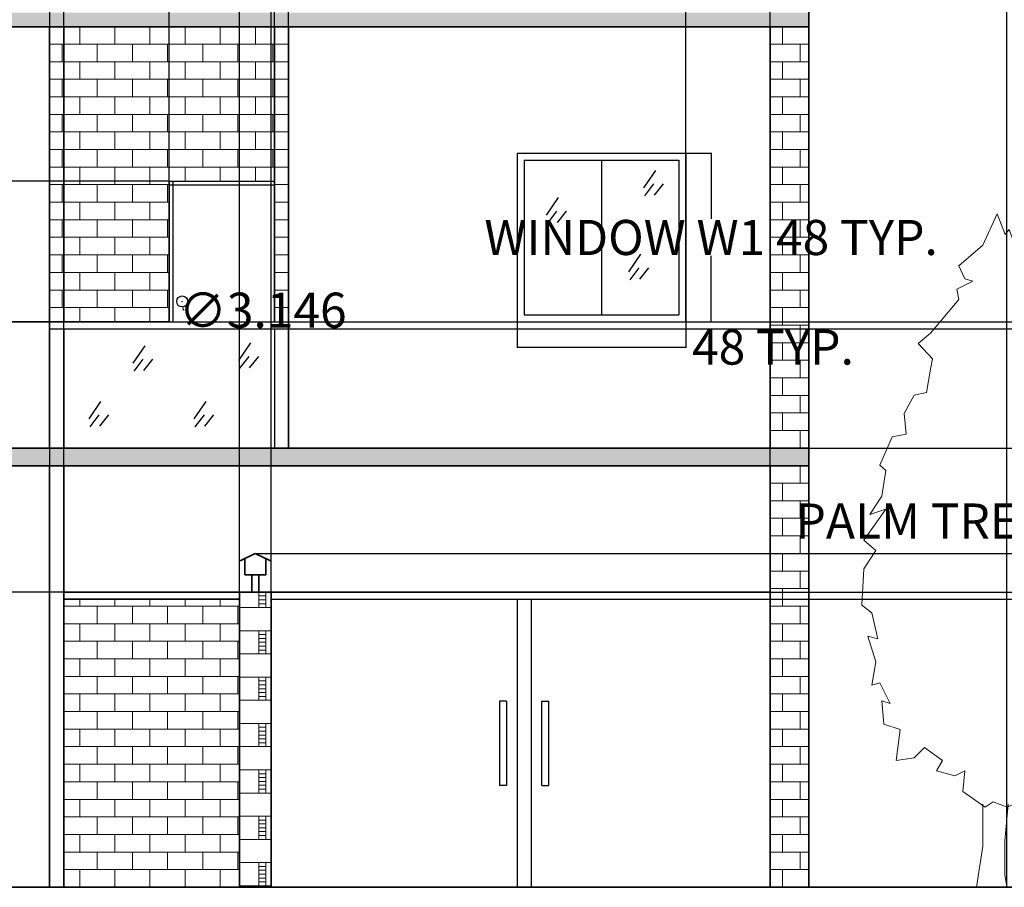
# Model space of a CAD drawing. Units: inches. Extents: x 403 to 1256, y 451 to 842.
# Tile 2 of 4: x 818 to 1098, y 455 to 702. Entities that reach past the tile are written whole.
import ezdxf

# ---------------------------------------------------------------- set-up
doc = ezdxf.new("R2010")
doc.units = ezdxf.units.IN
doc.header["$MEASUREMENT"] = 0
for name, color, linetype, lineweight in [('A-ANNO-DIMS', 2, 'Continuous', 18), ('A-DOOR', 4, 'Continuous', 25), ('A-GLAZ', 4, 'Continuous', 25), ('A-WALL', 7, 'Continuous', 35), ('A-WALL-PATT', 8, 'Continuous', 13), ('PLANTS', 3, 'Continuous', 18)]:
    doc.layers.add(name, color=color, linetype=linetype, lineweight=lineweight)
doc.styles.get("Standard").update_dxf_attribs({"font": 'arial.ttf'})
doc.dimstyles.get("Standard").update_dxf_attribs({"dimtxt": 10, "dimasz": 0.18, "dimexe": 0.18, "dimexo": 0.0625, "dimgap": 0.09, "dimtad": 0, "dimtih": 1, "dimtoh": 1, "dimdec": 0, "dimzin": 0, "dimdsep": 46, "dimlunit": 3, "dimtxsty": 'Standard', "dimcen": 0.09, "dimadec": 0, "dimazin": 0, "dimtfac": 1, "dimtdec": 0, "dimtofl": 0, "dimtmove": 0, "dimatfit": 3, "dimfxl": 1, "dimtolj": 1, "dimtzin": 0, "dimarcsym": 0})
pattern_1 = [(50, (0, 0), (6.455342, -0.56477), [0.675, -7.425]), (355, (0, 0), (-1.248762, 6.76973), [0.54, -5.94]), (100.45144, (0.538, -0.047), (5.20658, 6.20496), [0.573662, -6.31028]), (46.1842, (0, 1.8), (9.60517, -1.489674), [1.0125, -11.1375]), (96.6356, (0.8, 1.676), (8.41196, 8.76707), [0.86049, -9.465424]), (351.1842, (0, 1.8), (8.41196, 8.76707), [0.81, -8.91]), (21, (0.9, 1.35), (5.372163, -3.62357), [0.675, -7.425]), (326, (0.9, 1.35), (2.189838, 6.52635), [0.54, -5.94]), (71.45144, (1.3477, 1.048), (7.562, 2.90278), [0.573662, -6.31028]), (37.5, (0, 0), (0.1094387, 2.9960447), [0, -5.868, 0, -6.03, 0, -5.9625]), (7.5, (0, 0), (2.367626, 3.549705), [0, -3.438, 0, -5.733, 0, -2.2725]), (327.5, (-2.007, 0), (4.804402, -0.202994), [0, -2.25, 0, -7.02, 0, -9.315]), (317.5, (-2.907, 0), (5.248676, 0.900945), [0, -2.925, 0, -4.662, 0, -6.615])]

# ---------------------------------------------------------------- blocks, each defined once
blk = doc.blocks.new('Tree - type 2 deciduous elevation')
blk.add_lwpolyline([(-2.754, 191.699), (-6.78, 182.851), (-13.682, 176.953), (-11.956, 173.266), (-9.656, 172.529), (-14.257, 170.317), (-13.682, 167.368), (-21.733, 157.783), (-25.184, 154.834), (-21.158, 150.41), (-21.733, 147.461), (-22.884, 140.825), (-26.334, 140.087), (-29.21, 134.926), (-28.635, 129.028), (-32.661, 128.291), (-36.111, 120.18), (-34.386, 118.706), (-35.536, 111.333), (-38.987, 106.171), (-34.386, 107.646), (-40.712, 98.798), (-37.261, 95.849), (-40.712, 90.688), (-41.287, 80.366), (-38.412, 78.154), (-36.686, 70.781), (-39.562, 71.518), (-37.261, 64.145), (-38.412, 57.509), (-36.111, 58.247), (-33.236, 52.348), (-35.536, 53.086), (-34.961, 46.45), (-30.36, 44.975), (-31.51, 36.128), (-26.334, 36.865), (-23.459, 39.814), (-18.283, 36.128), (-20.008, 33.178), (-14.832, 31.704), (-11.956, 33.178), (-12.531, 27.28), (-6.205, 22.856), (-3.905, 24.331), (0.121, 22.856), (8.173, 26.543), (11.624, 25.068), (12.199, 27.28), (21.4, 34.653), (19.675, 39.077), (23.701, 44.975), (30.027, 47.924), (30.602, 53.823), (25.426, 56.772), (32.903, 61.196), (34.053, 67.094), (30.602, 75.205), (34.628, 89.951), (26.576, 103.222), (23.701, 103.222), (28.302, 107.646), (23.701, 110.595), (26.576, 115.756), (25.426, 117.968), (20.825, 118.706), (24.276, 124.604), (22.551, 137.876), (19.1, 139.35), (22.551, 140.825), (19.675, 151.884), (14.499, 153.359), (16.224, 162.207), (12.199, 170.317), (10.473, 167.368), (5.872, 179.165), (4.147, 177.69), (0.696, 187.275), (-0.454, 185.8)], close=True)
for points in [[(-6.813, 23.669), (-6.813, 11.669), (-8.627, 0)], [(0.387, 23.669), (-0.576, 13.271), (-0.576, 3.686), (0, 0)]]:
    blk.add_lwpolyline(points)
blk = doc.blocks.new('WIN-1200')
for p, q in [((0, 48), (0, 0)), ((0, 48), (48, 48)), ((48, 48), (48, 0)), ((2, 46), (46, 46)), ((2, 46), (2, 2)), ((24, 46), (24, 2)), ((46, 46), (46, 2)), ((39.35, 43.11), (35.96, 38.1)), ((38.86, 39.23), (36.28, 35.84)), ((41.61, 39.23), (39.03, 36)), ((11.71, 35.36), (8.32, 30.35)), ((11.23, 31.48), (8.64, 28.09)), ((13.98, 31.48), (11.39, 28.25)), ((35.15, 19.21), (31.75, 14.2)), ((34.66, 15.33), (32.08, 11.94)), ((37.41, 15.33), (34.82, 12.1)), ((2, 2), (46, 2)), ((0, 0), (48, 0))]:
    blk.add_line(p, q)
blk = doc.blocks.new('DOOR-HANDLE')
for p, q in [((0, 24), (0, 0)), ((2, 24), (0, 24)), ((2, 24), (2, 0)), ((2, 0), (0, 0))]:
    blk.add_line(p, q)
blk = doc.blocks.new('*D5')
at = {"layer": 'A-ANNO-DIMS', "color": 0, "lineweight": -2, "transparency": 16777216}
for p, q in [((1007.52, 663.96), (1014.84, 663.96)), ((1014.66, 663.78), (1014.66, 645.23)), ((1014.66, 616.14), (1014.66, 634.7)), ((1007.52, 615.96), (1014.84, 615.96))]:
    blk.add_line(p, q, dxfattribs=at)
at = {"layer": 'A-ANNO-DIMS', "color": 0, "transparency": 16777216}
for points in [[(1014.63, 663.78), (1014.69, 663.78), (1014.66, 663.96)], [(1014.63, 616.14), (1014.69, 616.14), (1014.66, 615.96)]]:
    blk.add_solid(points, dxfattribs=at)
at = {"layer": 'Defpoints', "color": 0, "transparency": 16777216}
for p in [(1007.46, 663.96), (1014.66, 663.96), (1007.46, 615.96)]:
    blk.add_point(p, dxfattribs=at)
at = {"layer": 'A-ANNO-DIMS', "color": 0, "transparency": 16777216, "insert": (1014.66, 639.96), "char_height": 10, "attachment_point": 5}
blk.add_mtext('\\A1;WINDOW W1 48 TYP.', dxfattribs=at)
blk = doc.blocks.new('*D6')
at = {"layer": 'A-ANNO-DIMS', "color": 0, "lineweight": -2, "transparency": 16777216}
for p, q in [((959.46, 615.9), (959.46, 608.58)), ((1007.46, 615.9), (1007.46, 608.58)), ((959.64, 608.76), (1007.28, 608.76)), ((1007.46, 608.76), (1007.64, 608.76))]:
    blk.add_line(p, q, dxfattribs=at)
at = {"layer": 'A-ANNO-DIMS', "color": 0, "transparency": 16777216}
for points in [[(959.64, 608.79), (959.64, 608.73), (959.46, 608.76)], [(1007.28, 608.79), (1007.28, 608.73), (1007.46, 608.76)]]:
    blk.add_solid(points, dxfattribs=at)
at = {"layer": 'Defpoints', "color": 0, "transparency": 16777216}
for p in [(959.46, 615.96), (1007.46, 615.96), (1007.46, 608.76)]:
    blk.add_point(p, dxfattribs=at)
at = {"layer": 'A-ANNO-DIMS', "color": 0, "transparency": 16777216, "insert": (1032.27, 608.76), "char_height": 10, "attachment_point": 5}
blk.add_mtext('\\A1;48 TYP.', dxfattribs=at)
blk = doc.blocks.new('*D7')
at = {"layer": 'A-ANNO-DIMS', "color": 0, "lineweight": -2, "transparency": 16777216}
for p, q in [((1132.84, 659.81), (1102.54, 659.81)), ((1102.72, 659.63), (1102.72, 564.43)), ((1102.72, 458.83), (1102.72, 554.04)), ((1132.84, 458.65), (1102.54, 458.65))]:
    blk.add_line(p, q, dxfattribs=at)
at = {"layer": 'A-ANNO-DIMS', "color": 0, "transparency": 16777216}
for points in [[(1102.69, 659.63), (1102.75, 659.63), (1102.72, 659.81)], [(1102.69, 458.83), (1102.75, 458.83), (1102.72, 458.65)]]:
    blk.add_solid(points, dxfattribs=at)
at = {"layer": 'Defpoints', "color": 0, "transparency": 16777216}
for p in [(1102.72, 659.81), (1132.9, 659.81), (1132.9, 458.65)]:
    blk.add_point(p, dxfattribs=at)
at = {"layer": 'A-ANNO-DIMS', "color": 0, "transparency": 16777216, "insert": (1102.72, 559.23), "char_height": 10, "attachment_point": 5}
blk.add_mtext('\\A1;PALM TREE 201 TYP.', dxfattribs=at)
blk = doc.blocks.new('*D12')
at = {"layer": 'A-ANNO-DIMS', "color": 0, "lineweight": -2, "transparency": 16777216}
for p, q in [((966.02, 799.96), (1244.44, 799.96)), ((1244.26, 799.78), (1244.26, 632.66)), ((1244.26, 455.14), (1244.26, 622.26)), ((1042.52, 454.96), (1244.44, 454.96))]:
    blk.add_line(p, q, dxfattribs=at)
at = {"layer": 'A-ANNO-DIMS', "color": 0, "transparency": 16777216}
for points in [[(1244.23, 799.78), (1244.29, 799.78), (1244.26, 799.96)], [(1244.23, 455.14), (1244.29, 455.14), (1244.26, 454.96)]]:
    blk.add_solid(points, dxfattribs=at)
at = {"layer": 'Defpoints', "color": 0, "transparency": 16777216}
for p in [(965.96, 799.96), (1244.26, 799.96), (1042.46, 454.96)]:
    blk.add_point(p, dxfattribs=at)
at = {"layer": 'A-ANNO-DIMS', "color": 0, "transparency": 16777216, "insert": (1244.26, 627.46), "char_height": 10, "attachment_point": 5}
blk.add_mtext('\\A1;345', dxfattribs=at)
blk = doc.blocks.new('*D19')
at = {"layer": 'A-ANNO-DIMS', "color": 0, "lineweight": -2, "transparency": 16777216}
for p, q in [((754.4, 490.96), (473.5, 490.96)), ((473.68, 490.78), (473.68, 478.16)), ((473.68, 455.14), (473.68, 467.76)), ((826.4, 454.96), (473.5, 454.96))]:
    blk.add_line(p, q, dxfattribs=at)
at = {"layer": 'A-ANNO-DIMS', "color": 0, "transparency": 16777216}
for points in [[(473.65, 490.78), (473.71, 490.78), (473.68, 490.96)], [(473.65, 455.14), (473.71, 455.14), (473.68, 454.96)]]:
    blk.add_solid(points, dxfattribs=at)
at = {"layer": 'Defpoints', "color": 0, "transparency": 16777216}
for p in [(754.46, 490.96), (473.68, 454.96), (826.46, 454.96)]:
    blk.add_point(p, dxfattribs=at)
at = {"layer": 'A-ANNO-DIMS', "color": 0, "transparency": 16777216, "insert": (473.68, 472.96), "char_height": 10, "attachment_point": 5}
blk.add_mtext('\\A1;36', dxfattribs=at)
blk = doc.blocks.new('*D20')
at = {"layer": 'A-ANNO-DIMS', "color": 0, "lineweight": -2, "transparency": 16777216}
for p, q in [((706.52, 615.96), (1244.44, 615.96)), ((1244.26, 615.78), (1244.26, 603.16)), ((1244.26, 580.14), (1244.26, 592.76)), ((682.52, 579.96), (1244.44, 579.96))]:
    blk.add_line(p, q, dxfattribs=at)
at = {"layer": 'A-ANNO-DIMS', "color": 0, "transparency": 16777216}
for points in [[(1244.23, 615.78), (1244.29, 615.78), (1244.26, 615.96)], [(1244.23, 580.14), (1244.29, 580.14), (1244.26, 579.96)]]:
    blk.add_solid(points, dxfattribs=at)
at = {"layer": 'Defpoints', "color": 0, "transparency": 16777216}
for p in [(706.46, 615.96), (1244.26, 615.96), (682.46, 579.96)]:
    blk.add_point(p, dxfattribs=at)
at = {"layer": 'A-ANNO-DIMS', "color": 0, "transparency": 16777216, "insert": (1244.26, 597.96), "char_height": 10, "attachment_point": 5}
blk.add_mtext('\\A1;36', dxfattribs=at)
blk = doc.blocks.new('*D22')
at = {"layer": 'A-ANNO-DIMS', "color": 0, "lineweight": -2, "transparency": 16777216}
for p, q in [((1007.46, 616.02), (1007.46, 835.54)), ((1007.64, 835.36), (1017.67, 835.36)), ((1042.28, 835.36), (1032.25, 835.36)), ((1042.46, 704.02), (1042.46, 835.54))]:
    blk.add_line(p, q, dxfattribs=at)
at = {"layer": 'A-ANNO-DIMS', "color": 0, "transparency": 16777216}
for points in [[(1007.64, 835.39), (1007.64, 835.33), (1007.46, 835.36)], [(1042.28, 835.39), (1042.28, 835.33), (1042.46, 835.36)]]:
    blk.add_solid(points, dxfattribs=at)
at = {"layer": 'Defpoints', "color": 0, "transparency": 16777216}
for p in [(1042.46, 835.36), (1042.46, 703.96), (1007.46, 615.96)]:
    blk.add_point(p, dxfattribs=at)
at = {"layer": 'A-ANNO-DIMS', "color": 0, "transparency": 16777216, "insert": (1024.96, 835.36), "char_height": 10, "attachment_point": 5}
blk.add_mtext('\\A1;35', dxfattribs=at)
blk = doc.blocks.new('*D23')
at = {"layer": 'A-ANNO-DIMS', "color": 0, "lineweight": -2, "transparency": 16777216}
for p, q in [((682.46, 455.02), (682.46, 835.54)), ((682.64, 835.36), (743.81, 835.36)), ((826.28, 835.36), (765.1, 835.36)), ((826.46, 455.02), (826.46, 835.54))]:
    blk.add_line(p, q, dxfattribs=at)
at = {"layer": 'A-ANNO-DIMS', "color": 0, "transparency": 16777216}
for points in [[(682.64, 835.39), (682.64, 835.33), (682.46, 835.36)], [(826.28, 835.39), (826.28, 835.33), (826.46, 835.36)]]:
    blk.add_solid(points, dxfattribs=at)
at = {"layer": 'Defpoints', "color": 0, "transparency": 16777216}
for p in [(826.46, 835.36), (682.46, 454.96), (826.46, 454.96)]:
    blk.add_point(p, dxfattribs=at)
at = {"layer": 'A-ANNO-DIMS', "color": 0, "transparency": 16777216, "insert": (754.46, 835.36), "char_height": 10, "attachment_point": 5}
blk.add_mtext('\\A1;144', dxfattribs=at)
blk = doc.blocks.new('*D24')
at = {"layer": 'A-ANNO-DIMS', "color": 0, "lineweight": -2, "transparency": 16777216}
for p, q in [((830.46, 539.02), (830.46, 835.54)), ((830.64, 835.36), (848.22, 835.36)), ((880.28, 835.36), (862.69, 835.36)), ((880.46, 539.02), (880.46, 835.54))]:
    blk.add_line(p, q, dxfattribs=at)
at = {"layer": 'A-ANNO-DIMS', "color": 0, "transparency": 16777216}
for points in [[(830.64, 835.39), (830.64, 835.33), (830.46, 835.36)], [(880.28, 835.39), (880.28, 835.33), (880.46, 835.36)]]:
    blk.add_solid(points, dxfattribs=at)
at = {"layer": 'Defpoints', "color": 0, "transparency": 16777216}
for p in [(880.46, 835.36), (830.46, 538.96), (880.46, 538.96)]:
    blk.add_point(p, dxfattribs=at)
at = {"layer": 'A-ANNO-DIMS', "color": 0, "transparency": 16777216, "insert": (855.46, 835.36), "char_height": 10, "attachment_point": 5}
blk.add_mtext('\\A1;50', dxfattribs=at)
blk = doc.blocks.new('*D25')
at = {"layer": 'A-ANNO-DIMS', "color": 0, "lineweight": -2, "transparency": 16777216}
for p, q in [((889.46, 539.02), (889.46, 835.54)), ((889.64, 835.36), (949.84, 835.36)), ((1031.28, 835.36), (971.07, 835.36)), ((1031.46, 539.02), (1031.46, 835.54))]:
    blk.add_line(p, q, dxfattribs=at)
at = {"layer": 'A-ANNO-DIMS', "color": 0, "transparency": 16777216}
for points in [[(889.64, 835.39), (889.64, 835.33), (889.46, 835.36)], [(1031.28, 835.39), (1031.28, 835.33), (1031.46, 835.36)]]:
    blk.add_solid(points, dxfattribs=at)
at = {"layer": 'Defpoints', "color": 0, "transparency": 16777216}
for p in [(1031.46, 835.36), (889.46, 538.96), (1031.46, 538.96)]:
    blk.add_point(p, dxfattribs=at)
at = {"layer": 'A-ANNO-DIMS', "color": 0, "transparency": 16777216, "insert": (960.46, 835.36), "char_height": 10, "attachment_point": 5}
blk.add_mtext('\\A1;142', dxfattribs=at)
blk = doc.blocks.new('*D26')
at = {"layer": 'A-ANNO-DIMS', "color": 0, "lineweight": -2, "transparency": 16777216}
for p, q in [((880.46, 539.02), (880.46, 835.54)), ((880.64, 835.36), (881.58, 835.36)), ((889.28, 835.36), (888.34, 835.36)), ((889.46, 539.02), (889.46, 835.54))]:
    blk.add_line(p, q, dxfattribs=at)
at = {"layer": 'A-ANNO-DIMS', "color": 0, "transparency": 16777216}
for points in [[(880.64, 835.39), (880.64, 835.33), (880.46, 835.36)], [(889.28, 835.39), (889.28, 835.33), (889.46, 835.36)]]:
    blk.add_solid(points, dxfattribs=at)
at = {"layer": 'Defpoints', "color": 0, "transparency": 16777216}
for p in [(889.46, 835.36), (880.46, 538.96), (889.46, 538.96)]:
    blk.add_point(p, dxfattribs=at)
at = {"layer": 'A-ANNO-DIMS', "color": 0, "transparency": 16777216, "insert": (884.96, 835.36), "char_height": 10, "attachment_point": 5}
blk.add_mtext('\\A1;9', dxfattribs=at)
blk = doc.blocks.new('*D27')
at = {"layer": 'A-ANNO-DIMS', "color": 0, "lineweight": -2, "transparency": 16777216}
for p, q in [((1031.46, 455.02), (1031.46, 835.54)), ((1031.64, 835.36), (1042.28, 835.36)), ((1042.46, 455.02), (1042.46, 835.54)), ((1042.46, 835.36), (1042.64, 835.36))]:
    blk.add_line(p, q, dxfattribs=at)
at = {"layer": 'A-ANNO-DIMS', "color": 0, "transparency": 16777216}
for points in [[(1031.64, 835.39), (1031.64, 835.33), (1031.46, 835.36)], [(1042.28, 835.39), (1042.28, 835.33), (1042.46, 835.36)]]:
    blk.add_solid(points, dxfattribs=at)
at = {"layer": 'Defpoints', "color": 0, "transparency": 16777216}
for p in [(1042.46, 835.36), (1031.46, 454.96), (1042.46, 454.96)]:
    blk.add_point(p, dxfattribs=at)
at = {"layer": 'A-ANNO-DIMS', "color": 0, "transparency": 16777216, "insert": (1048.46, 835.36), "char_height": 10, "attachment_point": 5}
blk.add_mtext('\\A1;11', dxfattribs=at)
blk = doc.blocks.new('*D30')
at = {"layer": 'A-ANNO-DIMS', "color": 0, "lineweight": -2, "transparency": 16777216}
for p, q in [((1042.46, 455.02), (1042.46, 835.54)), ((1042.64, 835.36), (1053.63, 835.36)), ((1098.63, 835.36), (1087.63, 835.36)), ((1098.81, 455.02), (1098.81, 835.54))]:
    blk.add_line(p, q, dxfattribs=at)
at = {"layer": 'A-ANNO-DIMS', "color": 0, "transparency": 16777216}
for points in [[(1042.64, 835.39), (1042.64, 835.33), (1042.46, 835.36)], [(1098.63, 835.39), (1098.63, 835.33), (1098.81, 835.36)]]:
    blk.add_solid(points, dxfattribs=at)
at = {"layer": 'Defpoints', "color": 0, "transparency": 16777216}
for p in [(1098.81, 835.36), (1042.46, 454.96), (1098.81, 454.96)]:
    blk.add_point(p, dxfattribs=at)
at = {"layer": 'A-ANNO-DIMS', "color": 0, "transparency": 16777216, "insert": (1070.63, 835.36), "char_height": 10, "attachment_point": 5}
blk.add_mtext('\\A1;56.35', dxfattribs=at)
blk = doc.blocks.new('*D32')
at = {"layer": 'A-ANNO-DIMS', "color": 0, "lineweight": -2, "transparency": 16777216}
for p, q in [((1031.52, 536.96), (1244.44, 536.96)), ((1244.26, 536.78), (1244.26, 501.16)), ((1244.26, 455.14), (1244.26, 490.77)), ((1031.52, 454.96), (1244.44, 454.96))]:
    blk.add_line(p, q, dxfattribs=at)
at = {"layer": 'A-ANNO-DIMS', "color": 0, "transparency": 16777216}
for points in [[(1244.23, 536.78), (1244.29, 536.78), (1244.26, 536.96)], [(1244.23, 455.14), (1244.29, 455.14), (1244.26, 454.96)]]:
    blk.add_solid(points, dxfattribs=at)
at = {"layer": 'Defpoints', "color": 0, "transparency": 16777216}
for p in [(1031.46, 536.96), (1244.26, 536.96), (1031.46, 454.96)]:
    blk.add_point(p, dxfattribs=at)
at = {"layer": 'A-ANNO-DIMS', "color": 0, "transparency": 16777216, "insert": (1244.26, 495.96), "char_height": 10, "attachment_point": 5}
blk.add_mtext('\\A1;82', dxfattribs=at)
blk = doc.blocks.new('*D33')
at = {"layer": 'A-ANNO-DIMS', "color": 0, "lineweight": -2, "transparency": 16777216}
for p, q in [((830.4, 538.96), (473.5, 538.96)), ((473.68, 538.78), (473.68, 502.16)), ((473.68, 455.14), (473.68, 491.77)), ((830.4, 454.96), (473.5, 454.96))]:
    blk.add_line(p, q, dxfattribs=at)
at = {"layer": 'A-ANNO-DIMS', "color": 0, "transparency": 16777216}
for points in [[(473.65, 538.78), (473.71, 538.78), (473.68, 538.96)], [(473.65, 455.14), (473.71, 455.14), (473.68, 454.96)]]:
    blk.add_solid(points, dxfattribs=at)
at = {"layer": 'Defpoints', "color": 0, "transparency": 16777216}
for p in [(473.68, 538.96), (830.46, 538.96), (830.46, 454.96)]:
    blk.add_point(p, dxfattribs=at)
at = {"layer": 'A-ANNO-DIMS', "color": 0, "transparency": 16777216, "insert": (473.68, 496.96), "char_height": 10, "attachment_point": 5}
blk.add_mtext('\\A1;84', dxfattribs=at)
blk = doc.blocks.new('*D34')
at = {"layer": 'A-ANNO-DIMS', "color": 0, "lineweight": -2, "transparency": 16777216}
for p, q in [((885.02, 549.96), (1244.44, 549.96)), ((1244.26, 549.78), (1244.26, 549.57)), ((886.02, 538.96), (1244.44, 538.96)), ((1244.26, 539.14), (1244.26, 539.35))]:
    blk.add_line(p, q, dxfattribs=at)
at = {"layer": 'A-ANNO-DIMS', "color": 0, "transparency": 16777216}
for points in [[(1244.23, 549.78), (1244.29, 549.78), (1244.26, 549.96)], [(1244.23, 539.14), (1244.29, 539.14), (1244.26, 538.96)]]:
    blk.add_solid(points, dxfattribs=at)
at = {"layer": 'Defpoints', "color": 0, "transparency": 16777216}
for p in [(884.96, 549.96), (1244.26, 549.96), (885.96, 538.96)]:
    blk.add_point(p, dxfattribs=at)
at = {"layer": 'A-ANNO-DIMS', "color": 0, "transparency": 16777216, "insert": (1244.26, 544.46), "char_height": 10, "attachment_point": 5}
blk.add_mtext('\\A1;11', dxfattribs=at)
blk = doc.blocks.new('*D35')
at = {"layer": 'A-ANNO-DIMS', "color": 0, "lineweight": -2, "transparency": 16777216}
for p, q in [((826.46, 616.02), (826.46, 835.54)), ((826.64, 835.36), (830.28, 835.36)), ((830.46, 616.02), (830.46, 835.54)), ((830.46, 835.36), (830.64, 835.36))]:
    blk.add_line(p, q, dxfattribs=at)
at = {"layer": 'A-ANNO-DIMS', "color": 0, "transparency": 16777216}
for points in [[(826.64, 835.39), (826.64, 835.33), (826.46, 835.36)], [(830.28, 835.39), (830.28, 835.33), (830.46, 835.36)]]:
    blk.add_solid(points, dxfattribs=at)
at = {"layer": 'Defpoints', "color": 0, "transparency": 16777216}
for p in [(830.46, 835.36), (826.46, 615.96), (830.46, 615.96)]:
    blk.add_point(p, dxfattribs=at)
at = {"layer": 'A-ANNO-DIMS', "color": 0, "transparency": 16777216, "insert": (834.19, 835.36), "char_height": 10, "attachment_point": 5}
blk.add_mtext('\\A1;4', dxfattribs=at)
blk = doc.blocks.new('*D36')
at = {"layer": 'A-ANNO-DIMS', "color": 0, "lineweight": -2, "transparency": 16777216}
for p, q in [((830.46, 616.02), (830.46, 835.54)), ((830.64, 835.36), (838.23, 835.36)), ((860.28, 835.36), (852.69, 835.36)), ((860.46, 616.02), (860.46, 835.54))]:
    blk.add_line(p, q, dxfattribs=at)
at = {"layer": 'A-ANNO-DIMS', "color": 0, "transparency": 16777216}
for points in [[(830.64, 835.39), (830.64, 835.33), (830.46, 835.36)], [(860.28, 835.39), (860.28, 835.33), (860.46, 835.36)]]:
    blk.add_solid(points, dxfattribs=at)
at = {"layer": 'Defpoints', "color": 0, "transparency": 16777216}
for p in [(860.46, 835.36), (830.46, 615.96), (860.46, 615.96)]:
    blk.add_point(p, dxfattribs=at)
at = {"layer": 'A-ANNO-DIMS', "color": 0, "transparency": 16777216, "insert": (845.46, 835.36), "char_height": 10, "attachment_point": 5}
blk.add_mtext('\\A1;30', dxfattribs=at)
blk = doc.blocks.new('*D37')
at = {"layer": 'A-ANNO-DIMS', "color": 0, "lineweight": -2, "transparency": 16777216}
for p, q in [((860.46, 656.02), (860.46, 835.54)), ((860.64, 835.36), (868.23, 835.36)), ((890.28, 835.36), (882.69, 835.36)), ((890.46, 656.02), (890.46, 835.54))]:
    blk.add_line(p, q, dxfattribs=at)
at = {"layer": 'A-ANNO-DIMS', "color": 0, "transparency": 16777216}
for points in [[(860.64, 835.39), (860.64, 835.33), (860.46, 835.36)], [(890.28, 835.39), (890.28, 835.33), (890.46, 835.36)]]:
    blk.add_solid(points, dxfattribs=at)
at = {"layer": 'Defpoints', "color": 0, "transparency": 16777216}
for p in [(890.46, 835.36), (860.46, 655.96), (890.46, 655.96)]:
    blk.add_point(p, dxfattribs=at)
at = {"layer": 'A-ANNO-DIMS', "color": 0, "transparency": 16777216, "insert": (875.46, 835.36), "char_height": 10, "attachment_point": 5}
blk.add_mtext('\\A1;30', dxfattribs=at)
blk = doc.blocks.new('*D38')
at = {"layer": 'A-ANNO-DIMS', "color": 0, "lineweight": -2, "transparency": 16777216}
for p, q in [((890.46, 616.02), (890.46, 835.54)), ((890.64, 835.36), (894.28, 835.36)), ((894.46, 616.02), (894.46, 835.54)), ((894.46, 835.36), (894.64, 835.36))]:
    blk.add_line(p, q, dxfattribs=at)
at = {"layer": 'A-ANNO-DIMS', "color": 0, "transparency": 16777216}
for points in [[(890.64, 835.39), (890.64, 835.33), (890.46, 835.36)], [(894.28, 835.39), (894.28, 835.33), (894.46, 835.36)]]:
    blk.add_solid(points, dxfattribs=at)
at = {"layer": 'Defpoints', "color": 0, "transparency": 16777216}
for p in [(894.46, 835.36), (890.46, 615.96), (894.46, 615.96)]:
    blk.add_point(p, dxfattribs=at)
at = {"layer": 'A-ANNO-DIMS', "color": 0, "transparency": 16777216, "insert": (898.19, 835.36), "char_height": 10, "attachment_point": 5}
blk.add_mtext('\\A1;4', dxfattribs=at)
blk = doc.blocks.new('*D39')
at = {"layer": 'A-ANNO-DIMS', "color": 0, "lineweight": -2, "transparency": 16777216}
for p, q in [((860.4, 655.96), (473.5, 655.96)), ((473.68, 655.78), (473.68, 641.16)), ((473.68, 616.14), (473.68, 630.77)), ((860.4, 615.96), (473.5, 615.96))]:
    blk.add_line(p, q, dxfattribs=at)
at = {"layer": 'A-ANNO-DIMS', "color": 0, "transparency": 16777216}
for points in [[(473.65, 655.78), (473.71, 655.78), (473.68, 655.96)], [(473.65, 616.14), (473.71, 616.14), (473.68, 615.96)]]:
    blk.add_solid(points, dxfattribs=at)
at = {"layer": 'Defpoints', "color": 0, "transparency": 16777216}
for p in [(473.68, 655.96), (860.46, 655.96), (860.46, 615.96)]:
    blk.add_point(p, dxfattribs=at)
at = {"layer": 'A-ANNO-DIMS', "color": 0, "transparency": 16777216, "insert": (473.68, 635.96), "char_height": 10, "attachment_point": 5}
blk.add_mtext('\\A1;40', dxfattribs=at)
blk = doc.blocks.new('*D40')
at = {"layer": 'A-ANNO-DIMS', "color": 0, "lineweight": -2, "transparency": 16777216}
for p, q in [((894.52, 613.96), (1244.44, 613.96)), ((1244.26, 613.78), (1244.26, 602.16)), ((1244.26, 580.14), (1244.26, 591.76)), ((894.52, 579.96), (1244.44, 579.96))]:
    blk.add_line(p, q, dxfattribs=at)
at = {"layer": 'A-ANNO-DIMS', "color": 0, "transparency": 16777216}
for points in [[(1244.23, 613.78), (1244.29, 613.78), (1244.26, 613.96)], [(1244.23, 580.14), (1244.29, 580.14), (1244.26, 579.96)]]:
    blk.add_solid(points, dxfattribs=at)
at = {"layer": 'Defpoints', "color": 0, "transparency": 16777216}
for p in [(894.46, 613.96), (1244.26, 613.96), (894.46, 579.96)]:
    blk.add_point(p, dxfattribs=at)
at = {"layer": 'A-ANNO-DIMS', "color": 0, "transparency": 16777216, "insert": (1244.26, 596.96), "char_height": 10, "attachment_point": 5}
blk.add_mtext('\\A1;34', dxfattribs=at)
blk = doc.blocks.new('*D41')
at = {"layer": 'A-ANNO-DIMS', "color": 0, "lineweight": -2, "transparency": 16777216}
for p, q in [((894.52, 615.96), (1244.44, 615.96)), ((894.52, 613.96), (1244.44, 613.96)), ((1244.26, 615.96), (1244.26, 616.14)), ((1244.26, 616.14), (1244.44, 616.14)), ((1244.26, 614.14), (1244.26, 615.78))]:
    blk.add_line(p, q, dxfattribs=at)
at = {"layer": 'A-ANNO-DIMS', "color": 0, "transparency": 16777216}
for points in [[(1244.23, 615.78), (1244.29, 615.78), (1244.26, 615.96)], [(1244.23, 614.14), (1244.29, 614.14), (1244.26, 613.96)]]:
    blk.add_solid(points, dxfattribs=at)
at = {"layer": 'Defpoints', "color": 0, "transparency": 16777216}
for p in [(894.46, 615.96), (894.46, 613.96), (1244.26, 615.96)]:
    blk.add_point(p, dxfattribs=at)
at = {"layer": 'A-ANNO-DIMS', "color": 0, "transparency": 16777216, "insert": (1247.85, 616.14), "char_height": 10, "attachment_point": 5}
blk.add_mtext('\\A1;2', dxfattribs=at)
blk = doc.blocks.new('*D53')
at = {"layer": 'A-ANNO-DIMS', "color": 0, "lineweight": -2, "transparency": 16777216}
for p, q in [((864.09, 621.75), (864.27, 621.75)), ((864.18, 621.66), (864.18, 621.84)), ((864.52, 619.25), (864.42, 620.01)), ((864.7, 619.25), (864.52, 619.25))]:
    blk.add_line(p, q, dxfattribs=at)
at = {"layer": 'A-ANNO-DIMS', "color": 0, "transparency": 16777216}
blk.add_solid([(864.45, 620.01), (864.39, 620.01), (864.39, 620.19)], dxfattribs=at)
at = {"layer": 'Defpoints', "color": 0, "transparency": 16777216}
for p in [(863.97, 623.3), (864.39, 620.19)]:
    blk.add_point(p, dxfattribs=at)
at = {"layer": 'A-ANNO-DIMS', "color": 0, "transparency": 16777216, "insert": (887.1, 619.25), "char_height": 10, "attachment_point": 5}
blk.add_mtext('\\A1;∅3.146', dxfattribs=at)

msp = doc.modelspace()

# ---------------------------------------------------------------- hatches: boundary and pattern name
at = {"layer": 'A-WALL-PATT'}
h = msp.add_hatch(dxfattribs=at)
h.set_pattern_fill('BRICK', color=256, scale=20)
h.paths.add_polyline_path([(673.459, 703.9615), (682.459, 703.9615), (682.459, 739.9615), (673.459, 739.9615)])
h.paths.add_polyline_path([(682.459, 699.9615), (673.459, 699.9615), (673.459, 579.9615), (682.459, 579.9615)])
h.paths.add_polyline_path([(673.459, 454.9615), (682.459, 454.9615), (682.459, 574.9615), (673.459, 574.9615)])
h.paths.add_polyline_path([(1031.459, 579.9615), (1042.459, 579.9615), (1042.459, 615.9615), (1042.459, 699.9615), (1033.459, 699.9615), (1031.459, 699.9615)])
h = msp.add_hatch(dxfattribs=at)
h.set_pattern_fill('AR-CONC', color=256, scale=0.9)
h.set_pattern_definition(pattern_1)
h.paths.add_polyline_path([(673.459, 703.9615), (673.459, 699.9615), (1033.459, 699.9615), (1042.459, 699.9615), (1042.459, 703.9615), (1033.459, 703.9615)])
h = msp.add_hatch(dxfattribs=at)
h.set_pattern_fill('BRICK', color=256, scale=20)
h.paths.add_polyline_path([(1042.459, 574.9615), (1031.459, 574.9615), (1031.459, 454.9615), (1042.459, 454.9615)])
h.paths.add_polyline_path([(890.459, 699.9615), (830.459, 699.9615), (830.459, 615.9615), (860.459, 615.9615), (860.459, 655.9615), (890.459, 655.9615)])
h.paths.add_polyline_path([(830.459, 699.9615), (826.459, 699.9615), (826.459, 615.9615), (830.459, 615.9615)])
h.paths.add_polyline_path([(894.459, 699.9615), (890.459, 699.9615), (890.459, 655.9615), (890.459, 615.9615), (894.459, 615.9615)])
h = msp.add_hatch(dxfattribs=at)
h.set_pattern_fill('AR-CONC', color=256, scale=0.9)
h.set_pattern_definition(pattern_1)
h.paths.add_polyline_path([(1042.459, 574.9615), (1042.459, 579.9615), (673.459, 579.9615), (673.459, 574.9615)])
h = msp.add_hatch(dxfattribs=at)
h.set_pattern_fill('BRSTONE', color=256, scale=20)
h.paths.add_polyline_path([(889.459, 538.9615), (880.459, 538.9615), (880.459, 454.9615), (889.459, 454.9615)])
h = msp.add_hatch(dxfattribs=at)
h.set_pattern_fill('BRICK', color=256, scale=20)
h.paths.add_polyline_path([(880.459, 536.9615), (830.459, 536.9615), (830.459, 454.9615), (880.459, 454.9615)])

# ---------------------------------------------------------------- linework, layer by layer
at = {"layer": 'A-DOOR'}
for p, q in [((860.459, 655.9615), (860.459, 615.9615)), ((860.459, 655.9615), (890.459, 655.9615)), ((861.459, 655.9615), (861.459, 615.9615)), ((860.459, 654.9615), (890.459, 654.9615)), ((889.459, 536.9615), (1031.459, 536.9615)), ((959.459, 536.9615), (959.459, 454.9615)), ((963.459, 536.9615), (963.459, 454.9615))]:
    msp.add_line(p, q, dxfattribs=at)
msp.add_circle((864.1801, 621.7463), 1.573, dxfattribs=at)
at = {"layer": 'A-GLAZ'}
for p, q in [((826.459, 615.9615), (894.459, 615.9615)), ((826.459, 613.9615), (894.459, 613.9615)), ((830.459, 613.9615), (830.459, 579.9615)), ((890.459, 613.9615), (890.459, 579.9615)), ((853.4953, 609.1536), (850.1014, 604.1477)), ((883.583, 609.9867), (880.189, 604.9808)), ((853.0105, 605.2781), (850.4246, 601.887)), ((855.758, 605.2781), (853.1721, 602.0484)), ((883.0981, 606.1111), (880.5122, 602.72)), ((885.8456, 606.1111), (883.2597, 602.8815)), ((840.9524, 593.3119), (837.5585, 588.306)), ((870.8599, 593.3119), (867.466, 588.306)), ((840.4676, 589.4364), (837.8817, 586.0453)), ((843.2151, 589.4364), (840.6292, 586.2067)), ((870.3751, 589.4364), (867.7892, 586.0453)), ((873.1225, 589.4364), (870.5367, 586.2067))]:
    msp.add_line(p, q, dxfattribs=at)
at = {"layer": 'A-WALL'}
for p, q in [((1042.459, 615.9615), (1042.459, 759.3006)), ((1042.459, 703.9615), (1042.459, 699.9615)), ((673.459, 699.9615), (1033.459, 699.9615)), ((826.459, 699.9615), (826.459, 579.9615)), ((830.459, 699.9615), (830.459, 615.9615)), ((890.459, 699.9615), (890.459, 615.9615)), ((894.459, 699.9615), (894.459, 579.9615)), ((1031.459, 699.9615), (1031.459, 579.9615)), ((1033.459, 699.9615), (1042.459, 699.9615)), ((1042.459, 615.9615), (1042.459, 454.9615)), ((673.459, 579.9615), (1042.459, 579.9615)), ((673.459, 574.9615), (1042.459, 574.9615)), ((826.459, 574.9615), (826.459, 454.9615)), ((830.459, 574.9615), (830.459, 454.9615)), ((1031.459, 574.9615), (1031.459, 454.9615)), ((884.959, 549.9615), (880.6579, 547.9461)), ((884.959, 549.9615), (889.2601, 547.9461)), ((881.959, 543.9615), (881.959, 548.5558)), ((887.959, 543.9615), (887.959, 548.5558)), ((883.959, 543.9615), (881.959, 543.9615)), ((883.959, 543.9615), (885.959, 543.9615)), ((883.959, 538.9615), (883.959, 543.9615)), ((885.959, 538.9615), (885.959, 543.9615)), ((885.959, 543.9615), (887.959, 543.9615)), ((830.459, 538.9615), (1031.459, 538.9615)), ((880.459, 538.9615), (880.459, 454.9615)), ((880.459, 538.9615), (889.459, 538.9615)), ((880.459, 538.9615), (1031.459, 538.9615)), ((889.459, 538.9615), (889.459, 454.9615)), ((889.459, 538.9615), (889.459, 454.9615)), ((830.459, 536.9615), (880.459, 536.9615)), ((673.459, 454.9615), (1042.459, 454.9615)), ((1042.459, 454.9615), (1200.0763, 454.9615))]:
    msp.add_line(p, q, dxfattribs=at)

# ---------------------------------------------------------------- block references
at = {"layer": 'A-DOOR'}
msp.add_blockref('DOOR-HANDLE', (954.459, 483.962), dxfattribs=at)
at = {"layer": 'A-DOOR', "rotation": 180}
msp.add_blockref('DOOR-HANDLE', (968.459, 507.961), dxfattribs=at)
at = {"layer": 'A-GLAZ'}
msp.add_blockref('WIN-1200', (959.459, 615.962), dxfattribs=at)
at = {"layer": 'PLANTS'}
msp.add_blockref('Tree - type 2 deciduous elevation', (1098.8106, 454.9615), dxfattribs=at)

# ---------------------------------------------------------------- dimensions: what is measured, and where the dimension line sits
at = {"layer": 'A-ANNO-DIMS'}
for base, p1, p2, override, picture, middle in [((826.459, 835.3615), (682.459, 454.9615), (826.459, 454.9615), {"dimdec": 0, "dimlfac": 1, "dimrnd": 0, "dimzin": 0, "dimdsep": 46, "dimlunit": 2}, '*D23', (754.459, 835.3615)), ((830.459, 835.3615), (826.459, 615.9615), (830.459, 615.9615), {"dimdec": 0, "dimlfac": 1, "dimrnd": 0, "dimzin": 0, "dimdsep": 46, "dimlunit": 2}, '*D35', (834.1874, 835.3615)), ((880.459, 835.3615), (830.459, 538.9615), (880.459, 538.9615), {"dimdec": 0, "dimlfac": 1, "dimrnd": 0, "dimzin": 0, "dimdsep": 46, "dimlunit": 2}, '*D24', (855.459, 835.3615)), ((860.459, 835.3615), (830.459, 615.9615), (860.459, 615.9615), {"dimdec": 0, "dimlfac": 1, "dimrnd": 0, "dimzin": 0, "dimdsep": 46, "dimlunit": 2}, '*D36', (845.459, 835.3615)), ((890.459, 835.3615), (860.459, 655.9615), (890.459, 655.9615), {"dimdec": 0, "dimlfac": 1, "dimrnd": 0, "dimzin": 0, "dimdsep": 46, "dimlunit": 2}, '*D37', (875.459, 835.3615)), ((889.459, 835.3615), (880.459, 538.9615), (889.459, 538.9615), {"dimdec": 0, "dimlfac": 1, "dimrnd": 0, "dimzin": 0, "dimdsep": 46, "dimlunit": 2}, '*D26', (884.959, 835.3615)), ((1031.459, 835.3615), (889.459, 538.9615), (1031.459, 538.9615), {"dimdec": 0, "dimlfac": 1, "dimrnd": 0, "dimzin": 0, "dimdsep": 46, "dimlunit": 2}, '*D25', (960.459, 835.3615)), ((894.459, 835.3615), (890.459, 615.9615), (894.459, 615.9615), {"dimdec": 0, "dimlfac": 1, "dimrnd": 0, "dimzin": 0, "dimdsep": 46, "dimlunit": 2}, '*D38', (898.1874, 835.3615)), ((1042.459, 835.3615), (1007.459, 615.9615), (1042.459, 703.9615), {"dimdec": 0, "dimlfac": 1, "dimrnd": 0, "dimzin": 0, "dimdsep": 46, "dimlunit": 2}, '*D22', (1024.959, 835.3615)), ((1042.459, 835.3615), (1031.459, 454.9615), (1042.459, 454.9615), {"dimdec": 0, "dimlfac": 1, "dimrnd": 0, "dimzin": 0, "dimdsep": 46, "dimlunit": 2}, '*D27', (1048.4555, 835.3615)), ((1098.8106, 835.3615), (1042.459, 454.9615), (1098.8106, 454.9615), {"dimdec": 2, "dimlfac": 1, "dimrnd": 0, "dimzin": 0, "dimdsep": 46, "dimlunit": 2}, '*D30', (1070.6348, 835.3615))]:
    dim = msp.add_linear_dim(base=base, p1=p1, p2=p2, dimstyle='Standard', override=override, dxfattribs=at)
    dim.commit()
    dim.dimension.update_dxf_attribs({"geometry": picture, "text_midpoint": middle})
for base, p1, p2, picture, middle in [((1244.264, 799.9615), (1042.459, 454.9615), (965.959, 799.9615), '*D12', (1244.264, 627.4615)), ((473.6816, 655.9615), (860.459, 615.9615), (860.459, 655.9615), '*D39', (473.6816, 635.9615)), ((1244.264, 615.9615), (894.459, 613.9615), (894.459, 615.9615), '*D41', (1247.8458, 616.1415)), ((1244.264, 615.9615), (682.459, 579.9615), (706.459, 615.9615), '*D20', (1244.264, 597.9615)), ((1244.264, 613.9615), (894.459, 579.9615), (894.459, 613.9615), '*D40', (1244.264, 596.9615)), ((1244.264, 549.9615), (885.959, 538.9615), (884.959, 549.9615), '*D34', (1244.264, 544.4615)), ((473.6816, 538.9615), (830.459, 454.9615), (830.459, 538.9615), '*D33', (473.6816, 496.9615)), ((1244.264, 536.9615), (1031.459, 454.9615), (1031.459, 536.9615), '*D32', (1244.264, 495.9615)), ((473.6816, 454.9615), (754.459, 490.9615), (826.459, 454.9615), '*D19', (473.6816, 472.9615))]:
    dim = msp.add_linear_dim(base=base, p1=p1, p2=p2, angle=90, dimstyle='Standard', override={"dimdec": 0, "dimlfac": 1, "dimrnd": 0, "dimzin": 0, "dimdsep": 46, "dimlunit": 2}, dxfattribs=at)
    dim.commit()
    dim.dimension.update_dxf_attribs({"geometry": picture, "text_midpoint": middle})
for base, p1, p2, text, picture, middle in [((1014.659, 663.9615), (1007.459, 615.9615), (1007.459, 663.9615), 'WINDOW W1 <> TYP.', '*D5', (1014.659, 639.9615)), ((1102.7239, 659.8145), (1132.8989, 458.6475), (1132.8989, 659.8145), 'PALM TREE <> TYP.', '*D7', (1102.7239, 559.231))]:
    dim = msp.add_linear_dim(base=base, p1=p1, p2=p2, angle=90, text=text, dimstyle='Standard', override={"dimdec": 0, "dimlfac": 1, "dimrnd": 0, "dimzin": 0, "dimdsep": 46, "dimlunit": 2}, dxfattribs=at)
    dim.commit()
    dim.dimension.update_dxf_attribs({"geometry": picture, "text_midpoint": middle})
dim = msp.add_diameter_dim_2p(p1=(863.9676, 623.3049), p2=(864.3925, 620.1878), dimstyle='Standard', override={"dimdec": 3, "dimlfac": 1, "dimrnd": 0, "dimzin": 0, "dimdsep": 46, "dimlunit": 2}, dxfattribs=at)
dim.commit()
dim.dimension.update_dxf_attribs({"geometry": '*D53', "text_midpoint": (887.0989, 619.2526), "dimtype": 163})
dim = msp.add_linear_dim(base=(1007.459, 608.7615), p1=(959.459, 615.9615), p2=(1007.459, 615.9615), text='<> TYP.', dimstyle='Standard', override={"dimdec": 0, "dimlfac": 1, "dimrnd": 0, "dimzin": 0, "dimdsep": 46, "dimlunit": 2}, dxfattribs=at)
dim.commit()
dim.dimension.update_dxf_attribs({"geometry": '*D6', "text_midpoint": (1032.2686, 608.7615)})

doc.saveas('drawing.dxf')
